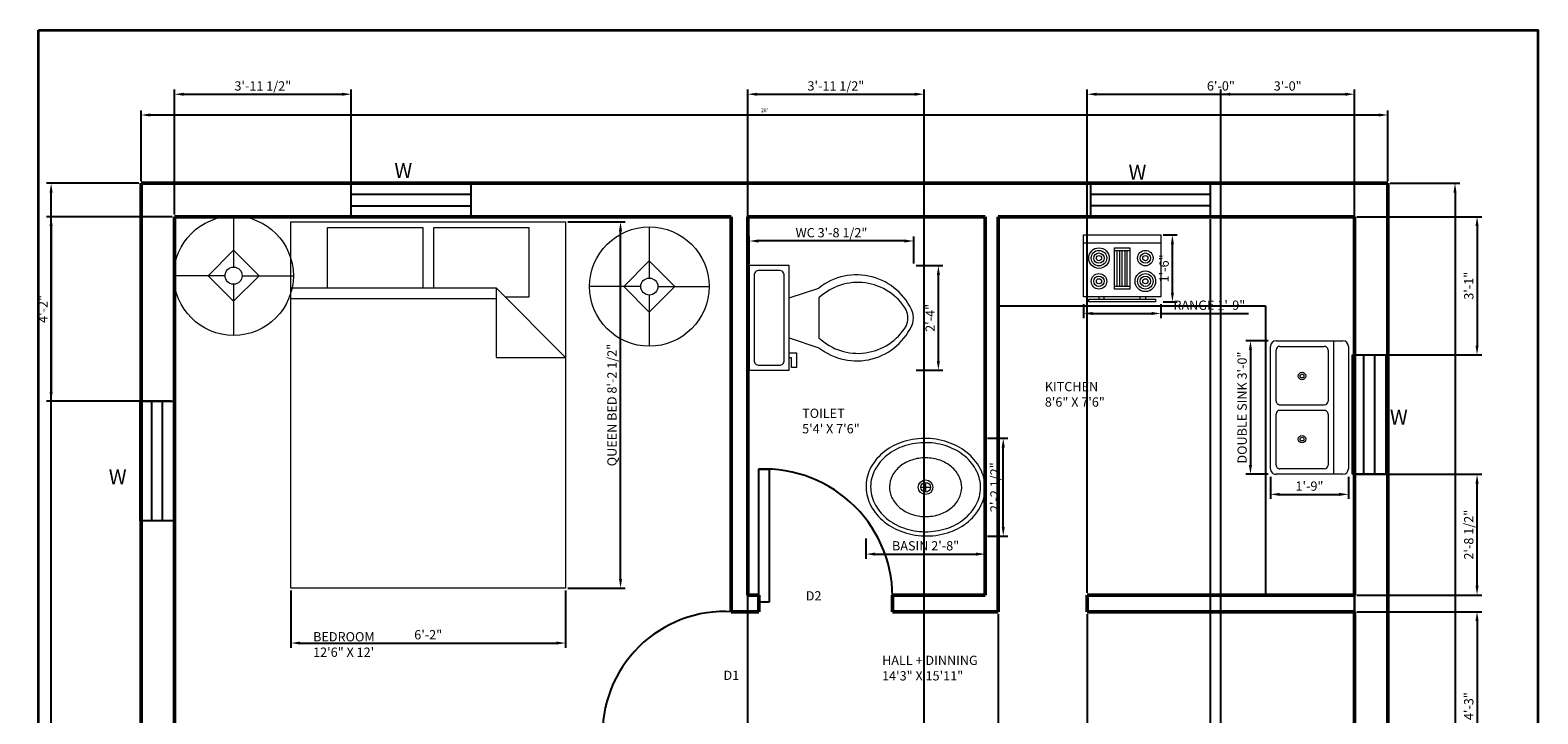
# Model space of a CAD drawing. Units: inches. Extents: x 216 to 622, y 47 to 588.
# Tile 3 of 3: x 216 to 622, y 403 to 588. Entities that reach past the tile are written whole.
import ezdxf

# ---------------------------------------------------------------- set-up
doc = ezdxf.new("R2010")
doc.units = ezdxf.units.IN
for name, color, linetype, lineweight in [('A-ANNO-TTLB', 7, 'Continuous', 35), ('A-AREA-IDEN', 7, 'Continuous', 18), ('A-DOOR', 3, 'Continuous', 25), ('A-EQPM', 8, 'Continuous', 18), ('A-FLOR-CASE', 8, 'Continuous', 25), ('A-FLOR-FIXT', 9, 'Continuous', 18), ('A-FURN', 8, 'Continuous', 18), ('A-GLAZ', 4, 'Continuous', 25), ('A-WALL', 7, 'Continuous', 50), ('Dimensions', 1, 'Continuous', 18), ('Text', 6, 'Continuous', 18)]:
    doc.layers.add(name, color=color, linetype=linetype, lineweight=lineweight)
doc.styles.get("Standard").update_dxf_attribs({"font": 'arial.ttf'})
doc.dimstyles.new('ISO-25', dxfattribs={"dimtxt": 2.5, "dimasz": 2.5, "dimexe": 1.25, "dimexo": 0.625, "dimtad": 1, "dimtxsty": 'Standard', "dimcen": 2.5, "dimadec": 0, "dimazin": 0, "dimtfac": 1, "dimtmove": 0, "dimatfit": 3, "dimfxl": 1, "dimarcsym": 0})

# ---------------------------------------------------------------- blocks, each defined once
blk = doc.blocks.new('Range-Oven - 30 in top')
for p, q in [((0, -3), (30, -3)), ((12, -6), (18, -6)), ((13, -20), (13, -6)), ((14, -6), (14, -20)), ((15, -20), (15, -6)), ((16, -6), (16, -20)), ((17, -20), (17, -6)), ((18, -20), (12, -20)), ((6, -24), (6, -25)), ((8, -25), (8, -24)), ((22, -25), (22, -24)), ((24, -24), (24, -25))]:
    blk.add_line(p, q)
for points in [[(0, -24), (0, 0), (30, 0), (30, -24)], [(12, -21), (12, -5), (18, -5), (18, -21)], [(2, -26), (2, -25), (28, -25), (28, -26)]]:
    blk.add_lwpolyline(points, close=True)
for centre, radius in [((6, -9), 4), ((6, -9), 3), ((6, -9), 2), ((6, -9), 1), ((24, -9), 3), ((24, -9), 2), ((24, -9), 1), ((6, -18), 3), ((6, -18), 2), ((6, -18), 1), ((24, -18), 4), ((24, -18), 3), ((24, -18), 2), ((24, -18), 1)]:
    blk.add_circle(centre, radius)
blk = doc.blocks.new('Sink-double - 36 in top')
for p, q in [((-18, -4), (18, -4)), ((-0.75, -18.5), (-0.75, -6.5)), ((0.75, -6.5), (0.75, -18.5))]:
    blk.add_line(p, q)
for points in [[(-16.5, 0), (16.5, 0)], [(-18, -19.5), (-18, -1.5)], [(18, -1.5), (18, -19.5)], [(-16.5, -18.5), (-16.5, -6.5)], [(-15.5, -5.5), (-1.75, -5.5)], [(1.75, -5.5), (15.5, -5.5)], [(16.5, -6.5), (16.5, -18.5)], [(-1.75, -19.5), (-15.5, -19.5)], [(15.5, -19.5), (1.75, -19.5)], [(16.5, -21), (-16.5, -21)]]:
    blk.add_lwpolyline(points)
for centre, radius in [((-8.5, -12.5), 1), ((-8.5, -12.5), 0.5), ((8.5, -12.5), 1), ((8.5, -12.5), 0.5)]:
    blk.add_circle(centre, radius)
for centre, radius, start, end in [((-16.5, -1.5), 1.5, 90, 180), ((16.5, -1.5), 1.5, 0, 90), ((-15.5, -6.5), 1, 90, 180), ((-1.75, -6.5), 1, 0, 90), ((1.75, -6.5), 1, 90, 180), ((15.5, -6.5), 1, 0, 90), ((-16.5, -19.5), 1.5, 180, 270), ((-15.5, -18.5), 1, 180, 270), ((-1.75, -18.5), 1, 270, 0), ((1.75, -18.5), 1, 180, 270), ((15.5, -18.5), 1, 270, 0), ((16.5, -19.5), 1.5, 270, 0)]:
    blk.add_arc(centre, radius, start, end)
blk = doc.blocks.new('Toilet - top')
for p, q in [((9.5, -6), (9.5, -2)), ((-10, -8.5), (-8, -8.5)), ((-10, -9.5), (-10, -8.5)), ((-8, -8.5), (-8, -8)), ((-7, -8), (-7, -9.5)), ((-4, -8), (-6, -14)), ((4, -8), (6, -14)), ((-7, -9.5), (-10, -9.5)), ((4, -14), (-4, -14))]:
    blk.add_line(p, q)
blk.add_lwpolyline([(10.5, -8), (10.5, 0), (-10.5, 0), (-10.5, -8)], close=True)
for points in [[(-9.5, -2), (-9.5, -6)], [(8.5, -1), (-8.5, -1)], [(-8.5, -7), (8.5, -7)]]:
    blk.add_lwpolyline(points)
for centre, radius, start, end in [((-8.62, -1.88), 0.884, 81.8699, 188.1301), ((8.62, -1.88), 0.884, 351.8699, 98.1301), ((-8.62, -6.12), 0.884, 171.8699, 278.1301), ((8.62, -6.12), 0.884, 261.8699, 8.1301), ((3.52, -21.58), 12.17, 141.4691, 247.9714), ((4.2, -21.82), 11.33, 136.3677, 238.9468), ((-3.52, -21.58), 12.17, 292.0284, 38.5307), ((-4.2, -21.82), 11.33, 301.053, 43.6321), ((0, -27.88), 4, 245.7318, 294.2682), ((0, -29), 4, 254.8605, 285.1395)]:
    blk.add_arc(centre, radius, start, end)
blk = doc.blocks.new('Bed - Queen')
for p, q in [((0, -80.00003), (0, 0)), ((0, 0), (59.99999, 0)), ((59.99999, 0), (59.99999, -80.00003)), ((7.99999, -1.2), (28.79998, -1.2)), ((7.99999, -14.4), (7.99999, -1.2)), ((28.79998, -1.2), (28.79998, -14.4)), ((31.19999, -1.2), (51.99999, -1.2)), ((31.19999, -14.4), (31.19999, -1.2)), ((51.99999, -1.2), (51.99999, -16.4)), ((0, -14.4), (44.8, -14.4)), ((59.99999, -29.6), (44.8, -14.4)), ((44.8, -14.4), (44.8, -29.6)), ((51.99999, -16.4), (46.79936, -16.4)), ((44.8, -16.8), (0, -16.8)), ((44.8, -29.6), (59.99999, -29.6)), ((59.99999, -80.00003), (0, -80.00003))]:
    blk.add_line(p, q)
blk = doc.blocks.new('Sink - Oval top')
for p, q in [((-1, 0), (1, 0)), ((0, 1), (0, -1))]:
    blk.add_line(p, q)
for points in [[(-12.23, 0.39, 0.117634), (-11.46, -3.36, 0.104469), (-8.88, -6.8, 0.090016), (-5.08, -9.07, 0.08192), (-0.32, -10.02, 0.08192), (4.49, -9.38, 0.090016), (8.42, -7.36, 0.104469), (11.22, -4.09, 0.117634), (12.23, -0.39, 0.117634), (11.46, 3.36, 0.104469), (8.88, 6.8, 0.090016), (5.08, 9.07, 0.08192), (0.32, 10.02, 0.08192), (-4.49, 9.38, 0.090016), (-8.42, 7.36, 0.104469), (-11.22, 4.09, 0.117634)], [(-11.29, 0.16, 0.118622), (-10.52, -3.25, 0.104678), (-8.07, -6.36, 0.089562), (-4.54, -8.37, 0.081185), (-0.13, -9.15, 0.081185), (4.3, -8.49, 0.089562), (7.89, -6.58, 0.104678), (10.42, -3.55, 0.118622), (11.29, -0.16, 0.118622), (10.52, 3.25, 0.104678), (8.07, 6.36, 0.089562), (4.54, 8.37, 0.081185), (0.13, 9.15, 0.081185), (-4.3, 8.49, 0.089562), (-7.89, 6.58, 0.104678), (-10.42, 3.55, 0.118622)], [(-7.42, 0.08, 0.118283), (-6.91, -2.17, 0.104607), (-5.29, -4.21, 0.089718), (-2.97, -5.53, 0.081436), (-0.07, -6.04, 0.081436), (2.84, -5.59, 0.089718), (5.2, -4.33, 0.104607), (6.86, -2.32, 0.118283), (7.42, -0.08, 0.118283), (6.91, 2.17, 0.104607), (5.29, 4.21, 0.089718), (2.97, 5.53, 0.081436), (0.07, 6.04, 0.081436), (-2.84, 5.59, 0.089718), (-5.2, 4.33, 0.104607), (-6.86, 2.32, 0.118283)]]:
    blk.add_lwpolyline(points, format="xyb", close=True)
for radius in [1.5, 1]:
    blk.add_circle((0, 0), radius)
blk = doc.blocks.new('Lamp - Table')
for p, q in [((0, 7), (0, 1)), ((0, 3), (-3, 0)), ((3, 0), (0, 3)), ((-1, 0), (-7, 0)), ((-3, 0), (0, -3)), ((0, -3), (3, 0)), ((1, 0), (7, 0)), ((0, -1), (0, -7))]:
    blk.add_line(p, q)
for radius in [7, 1]:
    blk.add_circle((0, 0), radius)
blk = doc.blocks.new('*D11')
at = {"layer": 'Defpoints', "color": 0, "transparency": 16777216}
for p in [(581.54, 564.89), (245.54, 546.47), (581.54, 546.47)]:
    blk.add_point(p, dxfattribs=at)
at = {"layer": 'Dimensions', "color": 0, "lineweight": -2, "transparency": 16777216}
for p, q in [((245.54, 547.09), (245.54, 566.14)), ((248.04, 564.89), (579.04, 564.89)), ((581.54, 547.09), (581.54, 566.14))]:
    blk.add_line(p, q, dxfattribs=at)
at = {"layer": 'Dimensions', "color": 0, "transparency": 16777216}
for points in [[(248.04, 565.3), (248.04, 564.47), (245.54, 564.89)], [(579.04, 565.3), (579.04, 564.47), (581.54, 564.89)]]:
    blk.add_solid(points, dxfattribs=at)
at = {"layer": 'Dimensions', "color": 0, "transparency": 16777216, "insert": (413.54, 566.02), "char_height": 1, "attachment_point": 5}
blk.add_mtext("28'", dxfattribs=at)
blk = doc.blocks.new('*D12')
at = {"layer": 'Defpoints', "color": 0, "transparency": 16777216}
for p in [(581.54, 546.47), (581.54, 90.47), (599.64, 90.47)]:
    blk.add_point(p, dxfattribs=at)
at = {"layer": 'Dimensions', "color": 0, "lineweight": -2, "transparency": 16777216}
for p, q in [((582.16, 546.47), (600.89, 546.47)), ((599.64, 543.97), (599.64, 92.97)), ((582.16, 90.47), (600.89, 90.47))]:
    blk.add_line(p, q, dxfattribs=at)
at = {"layer": 'Dimensions', "color": 0, "transparency": 16777216}
for points in [[(599.22, 543.97), (600.05, 543.97), (599.64, 546.47)], [(599.22, 92.97), (600.05, 92.97), (599.64, 90.47)]]:
    blk.add_solid(points, dxfattribs=at)
at = {"layer": 'Dimensions', "color": 0, "transparency": 16777216, "insert": (598.5, 318.47), "char_height": 1, "attachment_point": 5, "rotation": 90}
blk.add_mtext("38'", dxfattribs=at)
blk = doc.blocks.new('WINDOW-W-PLAN')
for p, q in [((0, 0), (0, 32.22)), ((0, 32.22), (9, 32.22)), ((3, 32.22), (3, 0)), ((6, 0), (6, 32.22)), ((9, 32.22), (9, 0)), ((9, 0), (0, 0))]:
    blk.add_line(p, q)
blk = doc.blocks.new('DOOR-PANEL-36IN-NOM')
blk.add_lwpolyline([(35.86, 2.79), (35.86, 0), (0, 0), (0, 2.79)], close=True)
blk = doc.blocks.new('*D23')
at = {"layer": 'Defpoints', "color": 0, "transparency": 16777216}
for p in [(359.94, 536.05), (374.75, 536.05), (359.94, 437.33)]:
    blk.add_point(p, dxfattribs=at)
at = {"layer": 'Dimensions', "color": 0, "lineweight": -2, "transparency": 16777216}
for p, q in [((360.57, 536.05), (376, 536.05)), ((374.75, 439.83), (374.75, 533.55)), ((360.57, 437.33), (376, 437.33))]:
    blk.add_line(p, q, dxfattribs=at)
at = {"layer": 'Dimensions', "color": 0, "transparency": 16777216}
for points in [[(374.33, 533.55), (375.17, 533.55), (374.75, 536.05)], [(374.33, 439.83), (375.17, 439.83), (374.75, 437.33)]]:
    blk.add_solid(points, dxfattribs=at)
at = {"layer": 'Dimensions', "color": 0, "transparency": 16777216, "insert": (372.76, 486.69), "char_height": 2.5, "attachment_point": 5, "rotation": 90}
blk.add_mtext('QUEEN BED 8\'-2 1/2"', dxfattribs=at)
blk = doc.blocks.new('*D24')
at = {"layer": 'Defpoints', "color": 0, "transparency": 16777216}
for p in [(285.91, 437.33), (359.94, 437.33), (359.94, 422.52)]:
    blk.add_point(p, dxfattribs=at)
at = {"layer": 'Dimensions', "color": 0, "lineweight": -2, "transparency": 16777216}
for p, q in [((285.91, 436.71), (285.91, 421.27)), ((359.94, 436.71), (359.94, 421.27)), ((288.41, 422.52), (357.44, 422.52))]:
    blk.add_line(p, q, dxfattribs=at)
at = {"layer": 'Dimensions', "color": 0, "transparency": 16777216}
for points in [[(288.41, 422.94), (288.41, 422.11), (285.91, 422.52)], [(357.44, 422.94), (357.44, 422.11), (359.94, 422.52)]]:
    blk.add_solid(points, dxfattribs=at)
at = {"layer": 'Dimensions', "color": 0, "transparency": 16777216, "insert": (322.92, 424.43), "char_height": 2.5, "attachment_point": 5}
blk.add_mtext('6\'-2"', dxfattribs=at)
blk = doc.blocks.new('*D27')
at = {"layer": 'Defpoints', "color": 0, "transparency": 16777216}
for p in [(409.44, 530.92), (409.44, 524.27), (453.76, 524.27)]:
    blk.add_point(p, dxfattribs=at)
at = {"layer": 'Dimensions', "color": 0, "lineweight": -2, "transparency": 16777216}
for p, q in [((409.44, 524.89), (409.44, 532.17)), ((451.26, 530.92), (411.94, 530.92)), ((453.76, 524.89), (453.76, 532.17))]:
    blk.add_line(p, q, dxfattribs=at)
at = {"layer": 'Dimensions', "color": 0, "transparency": 16777216}
for points in [[(411.94, 531.33), (411.94, 530.5), (409.44, 530.92)], [(451.26, 531.33), (451.26, 530.5), (453.76, 530.92)]]:
    blk.add_solid(points, dxfattribs=at)
at = {"layer": 'Dimensions', "color": 0, "transparency": 16777216, "insert": (431.6, 532.83), "char_height": 2.5, "attachment_point": 5}
blk.add_mtext('WC 3\'-8 1/2"', dxfattribs=at)
blk = doc.blocks.new('*D28')
at = {"layer": 'Defpoints', "color": 0, "transparency": 16777216}
for p in [(453.76, 524.27), (460.4, 524.27), (453.76, 496.1)]:
    blk.add_point(p, dxfattribs=at)
at = {"layer": 'Dimensions', "color": 0, "lineweight": -2, "transparency": 16777216}
for p, q in [((454.38, 524.27), (461.65, 524.27)), ((460.4, 498.6), (460.4, 521.77)), ((454.38, 496.1), (461.65, 496.1))]:
    blk.add_line(p, q, dxfattribs=at)
at = {"layer": 'Dimensions', "color": 0, "transparency": 16777216}
for points in [[(459.99, 521.77), (460.82, 521.77), (460.4, 524.27)], [(459.99, 498.6), (460.82, 498.6), (460.4, 496.1)]]:
    blk.add_solid(points, dxfattribs=at)
at = {"layer": 'Dimensions', "color": 0, "transparency": 16777216, "insert": (458.52, 510.19), "char_height": 2.5, "attachment_point": 5, "rotation": 90}
blk.add_mtext('2\'-4"', dxfattribs=at)
blk = doc.blocks.new('*D31')
at = {"layer": 'Defpoints', "color": 0, "transparency": 16777216}
for p in [(499.52, 514.5), (520.35, 514.5), (520.35, 511.38)]:
    blk.add_point(p, dxfattribs=at)
at = {"layer": 'Dimensions', "color": 0, "lineweight": -2, "transparency": 16777216}
for p, q in [((499.52, 513.88), (499.52, 510.13)), ((520.35, 513.88), (520.35, 510.13)), ((502.02, 511.38), (517.85, 511.38)), ((520.35, 511.38), (544, 511.38))]:
    blk.add_line(p, q, dxfattribs=at)
at = {"layer": 'Dimensions', "color": 0, "transparency": 16777216}
for points in [[(502.02, 511.79), (502.02, 510.96), (499.52, 511.38)], [(517.85, 511.79), (517.85, 510.96), (520.35, 511.38)]]:
    blk.add_solid(points, dxfattribs=at)
at = {"layer": 'Dimensions', "color": 0, "transparency": 16777216, "insert": (533.43, 513.29), "char_height": 2.5, "attachment_point": 5}
blk.add_mtext('RANGE 1\'-9"', dxfattribs=at)
blk = doc.blocks.new('*D32')
at = {"layer": 'Defpoints', "color": 0, "transparency": 16777216}
for p in [(520.35, 532.55), (523.47, 532.55), (520.35, 514.5)]:
    blk.add_point(p, dxfattribs=at)
at = {"layer": 'Dimensions', "color": 0, "lineweight": -2, "transparency": 16777216}
for p, q in [((520.97, 532.55), (524.72, 532.55)), ((523.47, 517), (523.47, 530.05)), ((520.97, 514.5), (524.72, 514.5))]:
    blk.add_line(p, q, dxfattribs=at)
at = {"layer": 'Dimensions', "color": 0, "transparency": 16777216}
for points in [[(523.06, 530.05), (523.89, 530.05), (523.47, 532.55)], [(523.06, 517), (523.89, 517), (523.47, 514.5)]]:
    blk.add_solid(points, dxfattribs=at)
at = {"layer": 'Dimensions', "color": 0, "transparency": 16777216, "insert": (521.57, 523.53), "char_height": 2.5, "attachment_point": 5, "rotation": 90}
blk.add_mtext('1\'-6"', dxfattribs=at)
blk = doc.blocks.new('*D33')
at = {"layer": 'Defpoints', "color": 0, "transparency": 16777216}
for p in [(549.91, 504.01), (544.51, 468.01), (549.91, 468.01)]:
    blk.add_point(p, dxfattribs=at)
at = {"layer": 'Dimensions', "color": 0, "lineweight": -2, "transparency": 16777216}
for p, q in [((549.28, 504.01), (543.26, 504.01)), ((544.51, 501.51), (544.51, 470.51)), ((549.28, 468.01), (543.26, 468.01))]:
    blk.add_line(p, q, dxfattribs=at)
at = {"layer": 'Dimensions', "color": 0, "transparency": 16777216}
for points in [[(544.09, 501.51), (544.92, 501.51), (544.51, 504.01)], [(544.09, 470.51), (544.92, 470.51), (544.51, 468.01)]]:
    blk.add_solid(points, dxfattribs=at)
at = {"layer": 'Dimensions', "color": 0, "transparency": 16777216, "insert": (542.59, 486.01), "char_height": 2.5, "attachment_point": 5, "rotation": 90}
blk.add_mtext('DOUBLE SINK 3\'-0"', dxfattribs=at)
blk = doc.blocks.new('*D34')
at = {"layer": 'Defpoints', "color": 0, "transparency": 16777216}
for p in [(549.91, 468.01), (570.91, 468.01), (570.91, 462.61)]:
    blk.add_point(p, dxfattribs=at)
at = {"layer": 'Dimensions', "color": 0, "lineweight": -2, "transparency": 16777216}
for p, q in [((549.91, 467.38), (549.91, 461.36)), ((570.91, 467.38), (570.91, 461.36)), ((552.41, 462.61), (568.41, 462.61))]:
    blk.add_line(p, q, dxfattribs=at)
at = {"layer": 'Dimensions', "color": 0, "transparency": 16777216}
for points in [[(552.41, 463.03), (552.41, 462.19), (549.91, 462.61)], [(568.41, 463.03), (568.41, 462.19), (570.91, 462.61)]]:
    blk.add_solid(points, dxfattribs=at)
at = {"layer": 'Dimensions', "color": 0, "transparency": 16777216, "insert": (560.41, 464.51), "char_height": 2.5, "attachment_point": 5}
blk.add_mtext('1\'-9"', dxfattribs=at)
blk = doc.blocks.new('*D35')
at = {"layer": 'Defpoints', "color": 0, "transparency": 16777216}
for p in [(440.86, 451.33), (473.06, 451.33), (473.06, 446.5)]:
    blk.add_point(p, dxfattribs=at)
at = {"layer": 'Dimensions', "color": 0, "lineweight": -2, "transparency": 16777216}
for p, q in [((440.86, 450.71), (440.86, 445.25)), ((473.06, 450.71), (473.06, 445.25)), ((443.36, 446.5), (470.56, 446.5))]:
    blk.add_line(p, q, dxfattribs=at)
at = {"layer": 'Dimensions', "color": 0, "transparency": 16777216}
for points in [[(443.36, 446.92), (443.36, 446.09), (440.86, 446.5)], [(470.56, 446.92), (470.56, 446.09), (473.06, 446.5)]]:
    blk.add_solid(points, dxfattribs=at)
at = {"layer": 'Dimensions', "color": 0, "transparency": 16777216, "insert": (456.96, 448.42), "char_height": 2.5, "attachment_point": 5}
blk.add_mtext('BASIN 2\'-8"', dxfattribs=at)
blk = doc.blocks.new('*D36')
at = {"layer": 'Defpoints', "color": 0, "transparency": 16777216}
for p in [(473.06, 477.74), (477.89, 477.74), (473.06, 451.33)]:
    blk.add_point(p, dxfattribs=at)
at = {"layer": 'Dimensions', "color": 0, "lineweight": -2, "transparency": 16777216}
for p, q in [((473.68, 477.74), (479.14, 477.74)), ((477.89, 453.83), (477.89, 475.24)), ((473.68, 451.33), (479.14, 451.33))]:
    blk.add_line(p, q, dxfattribs=at)
at = {"layer": 'Dimensions', "color": 0, "transparency": 16777216}
for points in [[(477.47, 475.24), (478.31, 475.24), (477.89, 477.74)], [(477.47, 453.83), (478.31, 453.83), (477.89, 451.33)]]:
    blk.add_solid(points, dxfattribs=at)
at = {"layer": 'Dimensions', "color": 0, "transparency": 16777216, "insert": (475.97, 464.54), "char_height": 2.5, "attachment_point": 5, "rotation": 90}
blk.add_mtext('2\'-2 1/2"', dxfattribs=at)
blk = doc.blocks.new('*D46')
at = {"layer": 'Defpoints', "color": 0, "transparency": 16777216}
for p in [(302.17, 570.49), (254.54, 537.47), (302.17, 537.42)]:
    blk.add_point(p, dxfattribs=at)
at = {"layer": 'Dimensions', "color": 0, "lineweight": -2, "transparency": 16777216}
for p, q in [((254.54, 538.09), (254.54, 571.74)), ((257.04, 570.49), (299.67, 570.49)), ((302.17, 538.04), (302.17, 571.74))]:
    blk.add_line(p, q, dxfattribs=at)
at = {"layer": 'Dimensions', "color": 0, "transparency": 16777216}
for points in [[(257.04, 570.9), (257.04, 570.07), (254.54, 570.49)], [(299.67, 570.9), (299.67, 570.07), (302.17, 570.49)]]:
    blk.add_solid(points, dxfattribs=at)
at = {"layer": 'Dimensions', "color": 0, "transparency": 16777216, "insert": (278.35, 572.4), "char_height": 2.5, "attachment_point": 5}
blk.add_mtext('3\'-11 1/2"', dxfattribs=at)
blk = doc.blocks.new('*D47')
at = {"layer": 'Defpoints', "color": 0, "transparency": 16777216}
for p in [(533.67, 537.45), (572.54, 537.47), (533.67, 49.13)]:
    blk.add_point(p, dxfattribs=at)
at = {"layer": 'Dimensions', "color": 0, "lineweight": -2, "transparency": 16777216}
for p, q in [((533.67, 536.83), (533.67, 47.88)), ((572.54, 536.84), (572.54, 47.88)), ((570.04, 49.13), (536.17, 49.13))]:
    blk.add_line(p, q, dxfattribs=at)
at = {"layer": 'Dimensions', "color": 0, "transparency": 16777216}
for points in [[(536.17, 49.55), (536.17, 48.71), (533.67, 49.13)], [(570.04, 49.55), (570.04, 48.71), (572.54, 49.13)]]:
    blk.add_solid(points, dxfattribs=at)
at = {"layer": 'Dimensions', "color": 0, "transparency": 16777216, "insert": (553.1, 51.03), "char_height": 2.5, "attachment_point": 5}
blk.add_mtext('3\'-3"', dxfattribs=at)
blk = doc.blocks.new('*D51')
at = {"layer": 'Defpoints', "color": 0, "transparency": 16777216}
for p in [(254.54, 537.47), (221.29, 487.7), (254.31, 487.7)]:
    blk.add_point(p, dxfattribs=at)
at = {"layer": 'Dimensions', "color": 0, "lineweight": -2, "transparency": 16777216}
for p, q in [((253.91, 537.47), (220.04, 537.47)), ((221.29, 534.97), (221.29, 490.2)), ((253.69, 487.7), (220.04, 487.7))]:
    blk.add_line(p, q, dxfattribs=at)
at = {"layer": 'Dimensions', "color": 0, "transparency": 16777216}
for points in [[(220.88, 534.97), (221.71, 534.97), (221.29, 537.47)], [(220.88, 490.2), (221.71, 490.2), (221.29, 487.7)]]:
    blk.add_solid(points, dxfattribs=at)
at = {"layer": 'Dimensions', "color": 0, "transparency": 16777216, "insert": (219.41, 512.59), "char_height": 2.5, "attachment_point": 5, "rotation": 90}
blk.add_mtext('4\'-2"', dxfattribs=at)
blk = doc.blocks.new('*D53')
at = {"layer": 'Defpoints', "color": 0, "transparency": 16777216}
for p in [(572.54, 430.97), (572.51, 380.05), (605.57, 380.05)]:
    blk.add_point(p, dxfattribs=at)
at = {"layer": 'Dimensions', "color": 0, "lineweight": -2, "transparency": 16777216}
for p, q in [((573.16, 430.97), (606.82, 430.97)), ((605.57, 428.47), (605.57, 382.55)), ((573.13, 380.05), (606.82, 380.05))]:
    blk.add_line(p, q, dxfattribs=at)
at = {"layer": 'Dimensions', "color": 0, "transparency": 16777216}
for points in [[(605.16, 428.47), (605.99, 428.47), (605.57, 430.97)], [(605.16, 382.55), (605.99, 382.55), (605.57, 380.05)]]:
    blk.add_solid(points, dxfattribs=at)
at = {"layer": 'Dimensions', "color": 0, "transparency": 16777216, "insert": (603.67, 405.51), "char_height": 2.5, "attachment_point": 5, "rotation": 90}
blk.add_mtext('4\'-3"', dxfattribs=at)
blk = doc.blocks.new('*D54')
at = {"layer": 'Defpoints', "color": 0, "transparency": 16777216}
for p in [(572.54, 537.47), (572.01, 500.24), (605.57, 500.24)]:
    blk.add_point(p, dxfattribs=at)
at = {"layer": 'Dimensions', "color": 0, "lineweight": -2, "transparency": 16777216}
for p, q in [((573.16, 537.47), (606.82, 537.47)), ((605.57, 534.97), (605.57, 502.74)), ((572.63, 500.24), (606.82, 500.24))]:
    blk.add_line(p, q, dxfattribs=at)
at = {"layer": 'Dimensions', "color": 0, "transparency": 16777216}
for points in [[(605.16, 534.97), (605.99, 534.97), (605.57, 537.47)], [(605.16, 502.74), (605.99, 502.74), (605.57, 500.24)]]:
    blk.add_solid(points, dxfattribs=at)
at = {"layer": 'Dimensions', "color": 0, "transparency": 16777216, "insert": (603.67, 518.85), "char_height": 2.5, "attachment_point": 5, "rotation": 90}
blk.add_mtext('3\'-1"', dxfattribs=at)
blk = doc.blocks.new('*D62')
at = {"layer": 'Defpoints', "color": 0, "transparency": 16777216}
for p in [(456.54, 570.49), (409.04, 99.47), (456.54, 99.47)]:
    blk.add_point(p, dxfattribs=at)
at = {"layer": 'Dimensions', "color": 0, "lineweight": -2, "transparency": 16777216}
for p, q in [((409.04, 100.09), (409.04, 571.74)), ((411.54, 570.49), (454.04, 570.49)), ((456.54, 100.09), (456.54, 571.74))]:
    blk.add_line(p, q, dxfattribs=at)
at = {"layer": 'Dimensions', "color": 0, "transparency": 16777216}
for points in [[(411.54, 570.9), (411.54, 570.07), (409.04, 570.49)], [(454.04, 570.9), (454.04, 570.07), (456.54, 570.49)]]:
    blk.add_solid(points, dxfattribs=at)
at = {"layer": 'Dimensions', "color": 0, "transparency": 16777216, "insert": (432.79, 572.4), "char_height": 2.5, "attachment_point": 5}
blk.add_mtext('3\'-11 1/2"', dxfattribs=at)
blk = doc.blocks.new('*D63')
at = {"layer": 'Defpoints', "color": 0, "transparency": 16777216}
for p in [(476.54, 430.97), (500.54, 430.97), (500.54, 49.13)]:
    blk.add_point(p, dxfattribs=at)
at = {"layer": 'Dimensions', "color": 0, "lineweight": -2, "transparency": 16777216}
for p, q in [((476.54, 430.34), (476.54, 47.88)), ((500.54, 430.34), (500.54, 47.88)), ((479.04, 49.13), (498.04, 49.13))]:
    blk.add_line(p, q, dxfattribs=at)
at = {"layer": 'Dimensions', "color": 0, "transparency": 16777216}
for points in [[(479.04, 49.55), (479.04, 48.71), (476.54, 49.13)], [(498.04, 49.55), (498.04, 48.71), (500.54, 49.13)]]:
    blk.add_solid(points, dxfattribs=at)
at = {"layer": 'Dimensions', "color": 0, "transparency": 16777216, "insert": (488.54, 51.03), "char_height": 2.5, "attachment_point": 5}
blk.add_mtext('2\'-0"', dxfattribs=at)
blk = doc.blocks.new('*D64')
at = {"layer": 'Defpoints', "color": 0, "transparency": 16777216}
for p in [(221.29, 546.47), (245.54, 546.47), (405.72, 73.15)]:
    blk.add_point(p, dxfattribs=at)
at = {"layer": 'Dimensions', "color": 0, "lineweight": -2, "transparency": 16777216}
for p, q in [((244.91, 546.47), (220.04, 546.47)), ((221.29, 75.65), (221.29, 543.97)), ((405.09, 73.15), (220.04, 73.15))]:
    blk.add_line(p, q, dxfattribs=at)
at = {"layer": 'Dimensions', "color": 0, "transparency": 16777216}
for points in [[(220.88, 543.97), (221.71, 543.97), (221.29, 546.47)], [(220.88, 75.65), (221.71, 75.65), (221.29, 73.15)]]:
    blk.add_solid(points, dxfattribs=at)
at = {"layer": 'Dimensions', "color": 0, "transparency": 16777216, "insert": (219.37, 309.81), "char_height": 2.5, "attachment_point": 5, "rotation": 90}
blk.add_mtext('39\'-5 1/2"', dxfattribs=at)
blk = doc.blocks.new('*D65')
at = {"layer": 'Defpoints', "color": 0, "transparency": 16777216}
for p in [(572.54, 570.49), (536.55, 123.47), (572.54, 123.47)]:
    blk.add_point(p, dxfattribs=at)
at = {"layer": 'Dimensions', "color": 0, "lineweight": -2, "transparency": 16777216}
for p, q in [((536.55, 124.09), (536.55, 571.74)), ((539.05, 570.49), (570.04, 570.49)), ((572.54, 124.09), (572.54, 571.74))]:
    blk.add_line(p, q, dxfattribs=at)
at = {"layer": 'Dimensions', "color": 0, "transparency": 16777216}
for points in [[(539.05, 570.9), (539.05, 570.07), (536.55, 570.49)], [(570.04, 570.9), (570.04, 570.07), (572.54, 570.49)]]:
    blk.add_solid(points, dxfattribs=at)
at = {"layer": 'Dimensions', "color": 0, "transparency": 16777216, "insert": (554.54, 572.39), "char_height": 2.5, "attachment_point": 5}
blk.add_mtext('3\'-0"', dxfattribs=at)
blk = doc.blocks.new('*D66')
at = {"layer": 'Defpoints', "color": 0, "transparency": 16777216}
for p in [(572.54, 570.49), (500.54, 435.47), (572.54, 435.47)]:
    blk.add_point(p, dxfattribs=at)
at = {"layer": 'Dimensions', "color": 0, "lineweight": -2, "transparency": 16777216}
for p, q in [((500.54, 436.09), (500.54, 571.74)), ((503.04, 570.49), (570.04, 570.49)), ((572.54, 436.09), (572.54, 571.74))]:
    blk.add_line(p, q, dxfattribs=at)
at = {"layer": 'Dimensions', "color": 0, "transparency": 16777216}
for points in [[(503.04, 570.9), (503.04, 570.07), (500.54, 570.49)], [(570.04, 570.9), (570.04, 570.07), (572.54, 570.49)]]:
    blk.add_solid(points, dxfattribs=at)
at = {"layer": 'Dimensions', "color": 0, "transparency": 16777216, "insert": (536.54, 572.39), "char_height": 2.5, "attachment_point": 5}
blk.add_mtext('6\'-0"', dxfattribs=at)
blk = doc.blocks.new('*D67')
at = {"layer": 'Defpoints', "color": 0, "transparency": 16777216}
for p in [(572.01, 468.02), (605.57, 468.02), (572.54, 435.47)]:
    blk.add_point(p, dxfattribs=at)
at = {"layer": 'Dimensions', "color": 0, "lineweight": -2, "transparency": 16777216}
for p, q in [((572.63, 468.02), (606.82, 468.02)), ((605.57, 437.97), (605.57, 465.52)), ((573.16, 435.47), (606.82, 435.47))]:
    blk.add_line(p, q, dxfattribs=at)
at = {"layer": 'Dimensions', "color": 0, "transparency": 16777216}
for points in [[(605.16, 465.52), (605.99, 465.52), (605.57, 468.02)], [(605.16, 437.97), (605.99, 437.97), (605.57, 435.47)]]:
    blk.add_solid(points, dxfattribs=at)
at = {"layer": 'Dimensions', "color": 0, "transparency": 16777216, "insert": (603.66, 451.74), "char_height": 2.5, "attachment_point": 5, "rotation": 90}
blk.add_mtext('2\'-8 1/2"', dxfattribs=at)

msp = doc.modelspace()

# ---------------------------------------------------------------- linework, layer by layer
at = {"layer": 'A-ANNO-TTLB'}
msp.add_lwpolyline([(217.87, 587.77), (621.96, 587.77), (621.96, 66.45), (217.87, 66.45)], close=True, dxfattribs=at)
at = {"layer": 'A-DOOR'}
for centre, radius, start, end in [((413.48, 434.85), 34.58, 357.5012, 92.3757), ((402.83, 398.09), 32.93, 86.4001, 182.8834)]:
    msp.add_arc(centre, radius, start, end, dxfattribs=at)
at = {"layer": 'A-FLOR-CASE'}
for p, q in [((476.54, 513.47), (548.54, 513.47)), ((548.54, 513.47), (548.54, 435.47))]:
    msp.add_line(p, q, dxfattribs=at)
at = {"layer": 'A-WALL'}
for p, q in [((245.54, 90.47), (245.54, 546.47)), ((245.54, 546.47), (581.54, 546.47)), ((581.54, 546.47), (581.54, 90.47)), ((254.54, 537.47), (404.54, 537.47)), ((254.54, 393.47), (254.54, 537.47)), ((404.54, 430.97), (404.54, 537.47)), ((404.54, 430.97), (404.54, 537.47)), ((409.04, 435.47), (409.04, 537.47)), ((409.04, 435.47), (409.04, 537.47)), ((409.04, 537.47), (473.04, 537.47)), ((473.04, 435.47), (473.04, 537.47)), ((476.54, 537.47), (476.54, 430.97)), ((476.54, 537.47), (572.54, 537.47)), ((572.54, 537.47), (572.54, 435.47)), ((409.04, 435.47), (412.04, 435.47)), ((412.04, 430.97), (412.04, 435.47)), ((448.04, 430.97), (448.04, 435.47)), ((448.04, 435.47), (473.04, 435.47)), ((500.54, 435.47), (572.54, 435.47)), ((500.54, 435.47), (500.54, 430.97)), ((404.54, 430.97), (412.04, 430.97)), ((448.04, 430.97), (476.54, 430.97)), ((500.54, 430.97), (572.54, 430.97)), ((572.54, 430.97), (572.54, 239.97))]:
    msp.add_line(p, q, dxfattribs=at)

# ---------------------------------------------------------------- block references
at = {"layer": 'A-DOOR', "rotation": 270}
msp.add_blockref('DOOR-PANEL-36IN-NOM', (412.05, 469.4), dxfattribs=at)
at = {"layer": 'A-EQPM', "xscale": 0.6942153254126727, "yscale": 0.6942153254126727, "zscale": 0.6942153254126727}
msp.add_blockref('Range-Oven - 30 in top', (499.52, 532.55), dxfattribs=at)
at = {"layer": 'A-FLOR-FIXT', "xscale": 1.341130096924882, "yscale": 1.341130096924882, "zscale": 1.341130096924882, "rotation": 90}
msp.add_blockref('Toilet - top', (409.44, 510.19), dxfattribs=at)
at = {"layer": 'A-FLOR-FIXT', "rotation": 270}
msp.add_blockref('Sink-double - 36 in top', (570.91, 486.01), dxfattribs=at)
at = {"layer": 'A-FLOR-FIXT', "xscale": 1.311488018161687, "yscale": 1.311488018161687, "zscale": 1.311488018161687}
msp.add_blockref('Sink - Oval top', (456.96, 464.54), dxfattribs=at)
at = {"layer": 'A-FURN'}
for name, p, xscale, yscale, zscale in [('Lamp - Table', (270.48, 521.57), 2.299024098102729, 2.299024098102729, 2.299024098102729), ('Bed - Queen', (285.91, 536.05), 1.233944108136291, 1.233944108136291, 1.233944108136291), ('Lamp - Table', (382.51, 518.64), 2.299024098102729, 2.299024098102729, 2.299024098102729)]:
    msp.add_blockref(name, p, dxfattribs=dict(at, xscale=xscale, yscale=yscale, zscale=zscale))
at = {"layer": 'A-GLAZ'}
for p, rotation in [((302.17, 546.42), 270.0000000000004), ((501.45, 546.45), 269.9999999999999), ((581.01, 500.24), 180), ((254.31, 487.7), 180)]:
    msp.add_blockref('WINDOW-W-PLAN', p, dxfattribs=dict(at, rotation=rotation))

# ---------------------------------------------------------------- texts
at = {"layer": 'A-AREA-IDEN', "char_height": 2.5, "attachment_point": 1}
for s, width, insert in [('KITCHEN\\P8\'6" X 7\'6"', 25.8762, (489.09, 492.92)), ('TOILET\\P5\'4\' X 7\'6"', 17.3397, (423.69, 485.72)), ('BEDROOM\\P12\'6" X 12\'', 66.9579, (291.9, 425.47)), ('HALL + DINNING\\P14\'3" X 15\'11"', 63.9956, (445.23, 419.11))]:
    msp.add_mtext_dynamic_manual_height_columns(s, width=width, gutter_width=12.5, heights=[0], dxfattribs=dict(at, insert=insert))
at = {"layer": 'Text', "attachment_point": 1}
for s, width, gutter_width, insert, char_height in [('W', 20.8525, 20.07, (313.8, 551.91), 4.01), ('W', 20.8525, 20.07, (511.65, 551.47), 4.01), ('W', 20.8525, 20.07, (582.09, 485.42), 4.01), ('W', 20.8525, 20.07, (236.83, 469.34), 4.01), ('D2', 6.2451, 12.5, (424.66, 436.5), 2.5), ('D1', 5.1919, 12.5, (402.49, 415.07), 2.5)]:
    msp.add_mtext_dynamic_manual_height_columns(s, width=width, gutter_width=gutter_width, heights=[0], dxfattribs=dict(at, insert=insert, char_height=char_height))

# ---------------------------------------------------------------- dimensions: what is measured, and where the dimension line sits
at = {"layer": 'Dimensions'}
for base, p1, p2, override, picture, middle in [((302.17, 570.49), (254.54, 537.47), (302.17, 537.42), {"dimdec": 1, "dimlfac": 1, "dimrnd": 0, "dimzin": 1, "dimdsep": 46, "dimlunit": 4, "dimfrac": 2}, '*D46', (278.35, 572.4)), ((456.54, 570.49), (409.04, 99.47), (456.54, 99.47), {"dimdec": 1, "dimlfac": 1, "dimrnd": 0, "dimzin": 1, "dimdsep": 46, "dimlunit": 4, "dimfrac": 2}, '*D62', (432.79, 572.4)), ((572.54, 570.49), (500.54, 435.47), (572.54, 435.47), {"dimdec": 1, "dimlfac": 1, "dimrnd": 0, "dimzin": 1, "dimdsep": 46, "dimlunit": 4, "dimfrac": 2}, '*D66', (536.54, 572.39)), ((572.54, 570.49), (536.55, 123.47), (572.54, 123.47), {"dimdec": 1, "dimlfac": 1, "dimrnd": 0, "dimzin": 1, "dimdsep": 46, "dimlunit": 4, "dimfrac": 2}, '*D65', (554.54, 572.39)), ((581.54, 564.89), (245.54, 546.47), (581.54, 546.47), {"dimtxt": 1, "dimdec": 0, "dimlunit": 3, "dimclrd": 0, "dimclre": 0, "dimclrt": 0, "dimtdec": 0}, '*D11', (413.54, 566.02)), ((533.67, 49.13), (572.54, 537.47), (533.67, 537.45), {"dimdec": 1, "dimlfac": 1, "dimrnd": 0, "dimzin": 1, "dimdsep": 46, "dimlunit": 4, "dimfrac": 2}, '*D47', (553.1, 51.03)), ((570.91, 462.61), (549.91, 468.01), (570.91, 468.01), {"dimdec": 1, "dimlfac": 1, "dimrnd": 0, "dimzin": 1, "dimdsep": 46, "dimlunit": 4, "dimfrac": 2}, '*D34', (560.41, 464.51)), ((359.94, 422.52), (285.91, 437.33), (359.94, 437.33), {"dimdec": 1, "dimlfac": 1, "dimrnd": 0, "dimzin": 1, "dimdsep": 46, "dimlunit": 4, "dimfrac": 2}, '*D24', (322.92, 424.43)), ((500.54, 49.13), (476.54, 430.97), (500.54, 430.97), {"dimdec": 1, "dimlfac": 1, "dimrnd": 0, "dimzin": 1, "dimdsep": 46, "dimlunit": 4, "dimfrac": 2}, '*D63', (488.54, 51.03))]:
    dim = msp.add_linear_dim(base=base, p1=p1, p2=p2, dimstyle='ISO-25', override=override, dxfattribs=at)
    dim.commit()
    dim.dimension.update_dxf_attribs({"geometry": picture, "text_midpoint": middle})
for base, p1, p2, override, picture, middle in [((221.29, 546.47), (405.72, 73.15), (245.54, 546.47), {"dimdec": 1, "dimlfac": 1, "dimrnd": 0, "dimzin": 1, "dimdsep": 46, "dimlunit": 4, "dimfrac": 2}, '*D64', (219.37, 309.81)), ((599.64, 90.47), (581.54, 546.47), (581.54, 90.47), {"dimtxt": 1, "dimdec": 0, "dimlunit": 3, "dimclrd": 0, "dimclre": 0, "dimclrt": 0, "dimtdec": 0}, '*D12', (598.5, 318.47)), ((221.29, 487.7), (254.54, 537.47), (254.31, 487.7), {"dimdec": 1, "dimlfac": 1, "dimrnd": 0, "dimzin": 1, "dimdsep": 46, "dimlunit": 4, "dimfrac": 2}, '*D51', (219.41, 512.59)), ((605.57, 500.24), (572.54, 537.47), (572.01, 500.24), {"dimdec": 1, "dimlfac": 1, "dimrnd": 0, "dimzin": 1, "dimdsep": 46, "dimlunit": 4, "dimfrac": 2}, '*D54', (603.67, 518.85)), ((523.4718, 532.5499), (520.3478, 514.5004), (520.3478, 532.5499), {"dimdec": 1, "dimlfac": 1, "dimrnd": 0, "dimzin": 1, "dimdsep": 46, "dimlunit": 4, "dimfrac": 2}, '*D32', (521.5703, 523.5252)), ((460.4, 524.27), (453.76, 496.1), (453.76, 524.27), {"dimdec": 1, "dimlfac": 1, "dimrnd": 0, "dimzin": 1, "dimdsep": 46, "dimlunit": 4, "dimfrac": 2}, '*D28', (458.52, 510.19)), ((477.89, 477.74), (473.06, 451.33), (473.06, 477.74), {"dimdec": 1, "dimlfac": 1, "dimrnd": 0, "dimzin": 1, "dimdsep": 46, "dimlunit": 4, "dimfrac": 2}, '*D36', (475.97, 464.54)), ((605.574, 468.018), (572.5368, 435.4661), (572.0091, 468.018), {"dimdec": 1, "dimlfac": 1, "dimrnd": 0, "dimzin": 1, "dimdsep": 46, "dimlunit": 4, "dimfrac": 2}, '*D67', (603.6564, 451.7421)), ((605.57, 380.05), (572.54, 430.97), (572.51, 380.05), {"dimdec": 1, "dimlfac": 1, "dimrnd": 0, "dimzin": 1, "dimdsep": 46, "dimlunit": 4, "dimfrac": 2}, '*D53', (603.67, 405.51))]:
    dim = msp.add_linear_dim(base=base, p1=p1, p2=p2, angle=90, dimstyle='ISO-25', override=override, dxfattribs=at)
    dim.commit()
    dim.dimension.update_dxf_attribs({"geometry": picture, "text_midpoint": middle})
for base, p1, p2, angle, text, picture, middle in [((409.44, 530.92), (453.76, 524.27), (409.44, 524.27), 180, 'WC <>', '*D27', (431.6, 532.83)), ((374.75, 536.05), (359.94, 437.33), (359.94, 536.05), 90, 'QUEEN BED <>', '*D23', (372.76, 486.69)), ((544.51, 468.01), (549.91, 504.01), (549.91, 468.01), 270, 'DOUBLE SINK <>', '*D33', (542.59, 486.01))]:
    dim = msp.add_linear_dim(base=base, p1=p1, p2=p2, angle=angle, text=text, dimstyle='ISO-25', override={"dimdec": 1, "dimlfac": 1, "dimrnd": 0, "dimzin": 1, "dimdsep": 46, "dimlunit": 4, "dimfrac": 2}, dxfattribs=at)
    dim.commit()
    dim.dimension.update_dxf_attribs({"geometry": picture, "text_midpoint": middle})
for base, p1, p2, text, picture, middle in [((520.35, 511.38), (499.52, 514.5), (520.35, 514.5), 'RANGE <>', '*D31', (533.43, 513.29)), ((473.06, 446.5), (440.86, 451.33), (473.06, 451.33), 'BASIN <>', '*D35', (456.96, 448.42))]:
    dim = msp.add_linear_dim(base=base, p1=p1, p2=p2, text=text, dimstyle='ISO-25', override={"dimdec": 1, "dimlfac": 1, "dimrnd": 0, "dimzin": 1, "dimdsep": 46, "dimlunit": 4, "dimfrac": 2}, dxfattribs=at)
    dim.commit()
    dim.dimension.update_dxf_attribs({"geometry": picture, "text_midpoint": middle})

doc.saveas('drawing.dxf')
